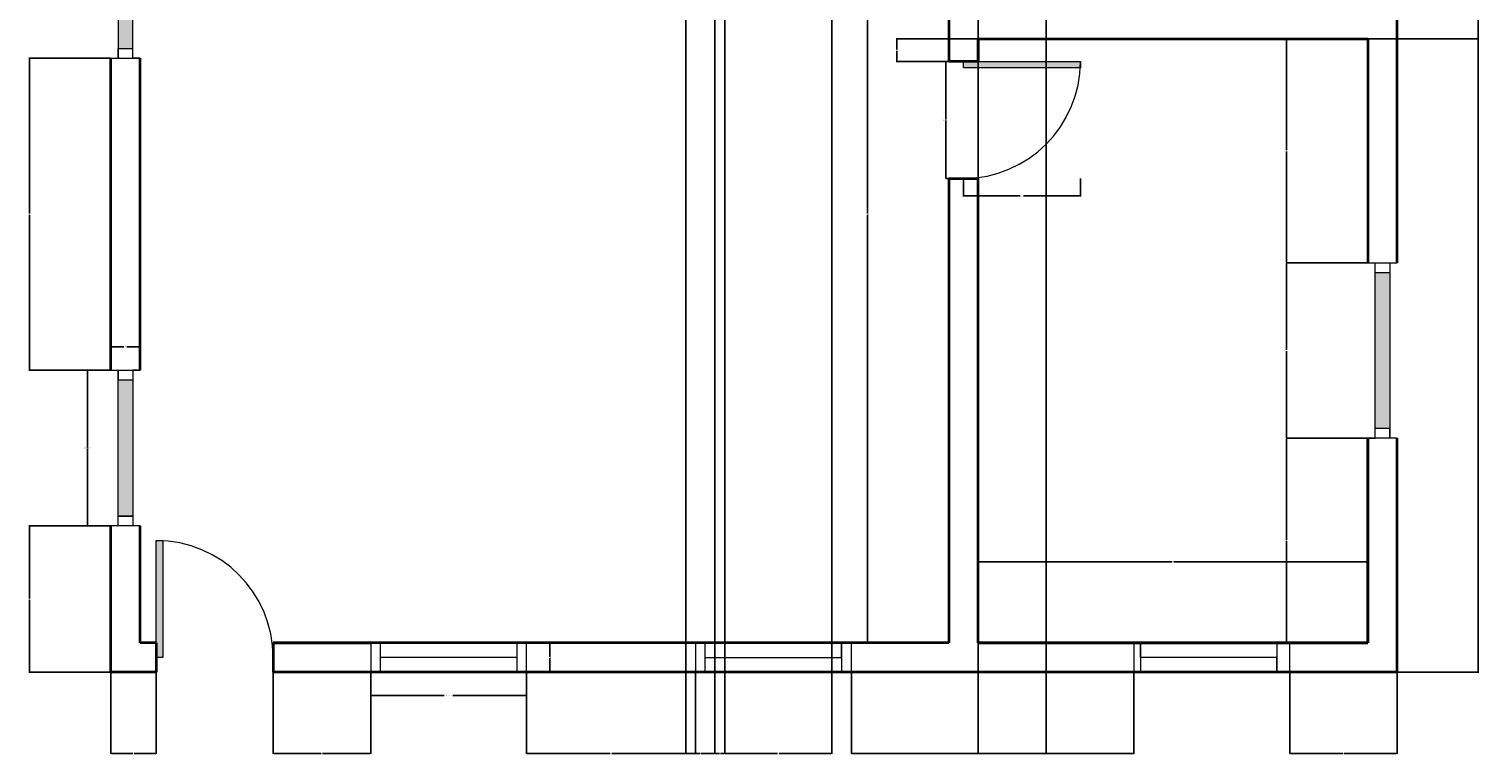
# Model space of a CAD drawing. Units: inches. Extents: x 2039 to 2485, y 1453 to 1986.
# Tile 1 of 4: x 2039 to 2485, y 1453 to 1676. Entities that reach past the tile are written whole.
import ezdxf

# ---------------------------------------------------------------- set-up
doc = ezdxf.new("R2010")
doc.units = ezdxf.units.IN
for name, color, linetype, lineweight in [('A-ANNO-DIMS', 2, 'Continuous', 18), ('A-DOOR', 3, 'Continuous', 18), ('A-GLAZ', 4, 'Continuous', 18), ('A-WALL', 7, 'Continuous', 35)]:
    doc.layers.add(name, color=color, linetype=linetype, lineweight=lineweight)
doc.layers.add('A-OPEN-PATT', color=18, linetype='Continuous', lineweight=13, true_color=0x000000)
doc.styles.get("Standard").update_dxf_attribs({"font": 'arial.ttf'})
doc.dimstyles.get("Standard").update_dxf_attribs({"dimtxt": 0.18, "dimasz": 0.18, "dimexe": 0.18, "dimexo": 0.0625, "dimgap": 0.09, "dimtad": 0, "dimtih": 1, "dimtoh": 1, "dimdec": 4, "dimzin": 0, "dimdsep": 46, "dimtxsty": 'Standard', "dimcen": 0.09, "dimadec": 0, "dimazin": 0, "dimtfac": 1, "dimtdec": 4, "dimtofl": 0, "dimtmove": 0, "dimatfit": 3, "dimfxl": 1, "dimtolj": 1, "dimtzin": 0, "dimarcsym": 0})

# ---------------------------------------------------------------- blocks, each defined once
blk = doc.blocks.new('DOOR-SWING-36IN')
for p, q in [((0, 0), (0, 36)), ((0, 36), (2, 36)), ((2, 36), (2, 0)), ((2, 0), (0, 0))]:
    blk.add_line(p, q)
blk.add_arc((0, 0), 36, 0, 90)
blk = doc.blocks.new('WIN-48IN')
for p, q in [((0, 48), (9, 48)), ((2.25, 3), (2.25, 48)), ((2.25, 48), (2.25, 45)), ((2.25, 45), (6.75, 45)), ((9, 48), (6.75, 48)), ((6.75, 48), (6.75, 0)), ((9, 0), (0, 0)), ((2.25, 0), (2.25, 3)), ((2.25, 3), (6.75, 3)), ((6.75, 3), (2.25, 3)), ((6.75, 0), (2.25, 0))]:
    blk.add_line(p, q)
blk = doc.blocks.new('WIN-48IN-CENTERLINE')
for p, q in [((0, 9), (0, 0)), ((3, 0), (3, 9)), ((45, 9), (45, 0)), ((48, 0), (48, 9)), ((45, 4.5), (3, 4.5))]:
    blk.add_line(p, q)
blk = doc.blocks.new('*D6')
at = {"layer": 'A-ANNO-DIMS', "color": 0, "lineweight": -2, "transparency": 16777216}
for p, q in [((2326.44, 1666.06), (2320.92, 1666.06)), ((2321.1, 1665.88), (2321.1, 1648.24)), ((2321.1, 1630.24), (2321.1, 1647.87)), ((2326.44, 1630.06), (2320.92, 1630.06))]:
    blk.add_line(p, q, dxfattribs=at)
at = {"layer": 'A-ANNO-DIMS', "color": 0, "transparency": 16777216}
for points in [[(2321.07, 1665.88), (2321.13, 1665.88), (2321.1, 1666.06)], [(2321.07, 1630.24), (2321.13, 1630.24), (2321.1, 1630.06)]]:
    blk.add_solid(points, dxfattribs=at)
at = {"layer": 'Defpoints', "color": 0, "transparency": 16777216}
for p in [(2326.5, 1666.06), (2321.1, 1630.06), (2326.5, 1630.06)]:
    blk.add_point(p, dxfattribs=at)
at = {"layer": 'A-ANNO-DIMS', "color": 0, "transparency": 16777216, "insert": (2321.1, 1648.06), "char_height": 0.18, "attachment_point": 5}
blk.add_mtext('\\A1;DOOR D1 36 TYP.', dxfattribs=at)
blk = doc.blocks.new('*D7')
at = {"layer": 'A-ANNO-DIMS', "color": 0, "lineweight": -2, "transparency": 16777216}
for p, q in [((2326.5, 1629.99), (2326.5, 1624.48)), ((2362.5, 1629.99), (2362.5, 1624.48)), ((2326.68, 1624.66), (2343.97, 1624.66)), ((2362.32, 1624.66), (2345.03, 1624.66))]:
    blk.add_line(p, q, dxfattribs=at)
at = {"layer": 'A-ANNO-DIMS', "color": 0, "transparency": 16777216}
for points in [[(2326.68, 1624.69), (2326.68, 1624.63), (2326.5, 1624.66)], [(2362.32, 1624.69), (2362.32, 1624.63), (2362.5, 1624.66)]]:
    blk.add_solid(points, dxfattribs=at)
at = {"layer": 'Defpoints', "color": 0, "transparency": 16777216}
for p in [(2326.5, 1630.06), (2362.5, 1630.06), (2362.5, 1624.66)]:
    blk.add_point(p, dxfattribs=at)
at = {"layer": 'A-ANNO-DIMS', "color": 0, "transparency": 16777216, "insert": (2344.5, 1624.66), "char_height": 0.18, "attachment_point": 5}
blk.add_mtext('\\A1;36 TYP.', dxfattribs=at)
blk = doc.blocks.new('*D12')
at = {"layer": 'A-ANNO-DIMS', "color": 0, "lineweight": -2, "transparency": 16777216}
for p, q in [((2063.94, 1571.06), (2056.62, 1571.06)), ((2056.8, 1570.88), (2056.8, 1547.24)), ((2056.8, 1523.24), (2056.8, 1546.87)), ((2063.94, 1523.06), (2056.62, 1523.06))]:
    blk.add_line(p, q, dxfattribs=at)
at = {"layer": 'A-ANNO-DIMS', "color": 0, "transparency": 16777216}
for points in [[(2056.77, 1570.88), (2056.83, 1570.88), (2056.8, 1571.06)], [(2056.77, 1523.24), (2056.83, 1523.24), (2056.8, 1523.06)]]:
    blk.add_solid(points, dxfattribs=at)
at = {"layer": 'Defpoints', "color": 0, "transparency": 16777216}
for p in [(2056.8, 1571.06), (2064, 1571.06), (2064, 1523.06)]:
    blk.add_point(p, dxfattribs=at)
at = {"layer": 'A-ANNO-DIMS', "color": 0, "transparency": 16777216, "insert": (2056.8, 1547.06), "char_height": 0.18, "attachment_point": 5}
blk.add_mtext('\\A1;WINDOW W2 48 TYP.', dxfattribs=at)
blk = doc.blocks.new('*D13')
at = {"layer": 'A-ANNO-DIMS', "color": 0, "lineweight": -2, "transparency": 16777216}
for p, q in [((2064, 1571.12), (2064, 1578.44)), ((2064.18, 1578.26), (2068.04, 1578.26)), ((2072.82, 1578.26), (2068.96, 1578.26)), ((2073, 1571.12), (2073, 1578.44))]:
    blk.add_line(p, q, dxfattribs=at)
at = {"layer": 'A-ANNO-DIMS', "color": 0, "transparency": 16777216}
for points in [[(2064.18, 1578.29), (2064.18, 1578.23), (2064, 1578.26)], [(2072.82, 1578.29), (2072.82, 1578.23), (2073, 1578.26)]]:
    blk.add_solid(points, dxfattribs=at)
at = {"layer": 'Defpoints', "color": 0, "transparency": 16777216}
for p in [(2073, 1578.26), (2064, 1571.06), (2073, 1571.06)]:
    blk.add_point(p, dxfattribs=at)
at = {"layer": 'A-ANNO-DIMS', "color": 0, "transparency": 16777216, "insert": (2068.5, 1578.26), "char_height": 0.18, "attachment_point": 5}
blk.add_mtext('\\A1;9 TYP.', dxfattribs=at)
blk = doc.blocks.new('*D14')
at = {"layer": 'A-ANNO-DIMS', "color": 0, "lineweight": -2, "transparency": 16777216}
for p, q in [((2144, 1477.99), (2144, 1470.68)), ((2192, 1477.99), (2192, 1470.68)), ((2144.18, 1470.86), (2166.66, 1470.86)), ((2191.82, 1470.86), (2169.34, 1470.86))]:
    blk.add_line(p, q, dxfattribs=at)
at = {"layer": 'A-ANNO-DIMS', "color": 0, "transparency": 16777216}
for points in [[(2144.18, 1470.89), (2144.18, 1470.83), (2144, 1470.86)], [(2191.82, 1470.89), (2191.82, 1470.83), (2192, 1470.86)]]:
    blk.add_solid(points, dxfattribs=at)
at = {"layer": 'Defpoints', "color": 0, "transparency": 16777216}
for p in [(2144, 1478.06), (2192, 1478.06), (2192, 1470.86)]:
    blk.add_point(p, dxfattribs=at)
at = {"layer": 'A-ANNO-DIMS', "color": 0, "transparency": 16777216, "insert": (2168, 1470.86), "char_height": 0.18, "attachment_point": 5}
blk.add_mtext('\\A1;WINDOW W3 48 TYP.', dxfattribs=at)
blk = doc.blocks.new('*D15')
at = {"layer": 'A-ANNO-DIMS', "color": 0, "lineweight": -2, "transparency": 16777216}
for p, q in [((2192.06, 1487.06), (2199.38, 1487.06)), ((2199.2, 1486.88), (2199.2, 1482.74)), ((2199.2, 1478.24), (2199.2, 1482.37)), ((2192.06, 1478.06), (2199.38, 1478.06))]:
    blk.add_line(p, q, dxfattribs=at)
at = {"layer": 'A-ANNO-DIMS', "color": 0, "transparency": 16777216}
for points in [[(2199.17, 1486.88), (2199.23, 1486.88), (2199.2, 1487.06)], [(2199.17, 1478.24), (2199.23, 1478.24), (2199.2, 1478.06)]]:
    blk.add_solid(points, dxfattribs=at)
at = {"layer": 'Defpoints', "color": 0, "transparency": 16777216}
for p in [(2192, 1487.06), (2199.2, 1487.06), (2192, 1478.06)]:
    blk.add_point(p, dxfattribs=at)
at = {"layer": 'A-ANNO-DIMS', "color": 0, "transparency": 16777216, "insert": (2199.2, 1482.56), "char_height": 0.18, "attachment_point": 5}
blk.add_mtext('\\A1;9 TYP.', dxfattribs=at)
blk = doc.blocks.new('*D17')
at = {"layer": 'A-ANNO-DIMS', "color": 0, "lineweight": -2, "transparency": 16777216}
for p, q in [((2460.06, 1961.06), (2485.19, 1961.06)), ((2485.01, 1960.88), (2485.01, 1719.74)), ((2485.01, 1478.24), (2485.01, 1719.37)), ((2460.06, 1478.06), (2485.19, 1478.06))]:
    blk.add_line(p, q, dxfattribs=at)
at = {"layer": 'A-ANNO-DIMS', "color": 0, "transparency": 16777216}
for points in [[(2484.98, 1960.88), (2485.04, 1960.88), (2485.01, 1961.06)], [(2484.98, 1478.24), (2485.04, 1478.24), (2485.01, 1478.06)]]:
    blk.add_solid(points, dxfattribs=at)
at = {"layer": 'Defpoints', "color": 0, "transparency": 16777216}
for p in [(2460, 1961.06), (2460, 1478.06), (2485.01, 1478.06)]:
    blk.add_point(p, dxfattribs=at)
at = {"layer": 'A-ANNO-DIMS', "color": 0, "transparency": 16777216, "insert": (2485.01, 1719.56), "char_height": 0.18, "attachment_point": 5}
blk.add_mtext('\\A1;483', dxfattribs=at)
blk = doc.blocks.new('*D20')
at = {"layer": 'A-ANNO-DIMS', "color": 0, "lineweight": -2, "transparency": 16777216}
for p, q in [((2064, 1477.99), (2064, 1452.87)), ((2078, 1477.99), (2078, 1452.87)), ((2064.18, 1453.05), (2070.79, 1453.05)), ((2077.82, 1453.05), (2071.21, 1453.05))]:
    blk.add_line(p, q, dxfattribs=at)
at = {"layer": 'A-ANNO-DIMS', "color": 0, "transparency": 16777216}
for points in [[(2064.18, 1453.08), (2064.18, 1453.02), (2064, 1453.05)], [(2077.82, 1453.08), (2077.82, 1453.02), (2078, 1453.05)]]:
    blk.add_solid(points, dxfattribs=at)
at = {"layer": 'Defpoints', "color": 0, "transparency": 16777216}
for p in [(2064, 1478.06), (2078, 1478.06), (2078, 1453.05)]:
    blk.add_point(p, dxfattribs=at)
at = {"layer": 'A-ANNO-DIMS', "color": 0, "transparency": 16777216, "insert": (2071, 1453.05), "char_height": 0.18, "attachment_point": 5}
blk.add_mtext('\\A1;14', dxfattribs=at)
blk = doc.blocks.new('*D21')
at = {"layer": 'A-ANNO-DIMS', "color": 0, "lineweight": -2, "transparency": 16777216}
for p, q in [((2114, 1477.99), (2114, 1452.87)), ((2144, 1477.99), (2144, 1452.87)), ((2114.18, 1453.05), (2128.78, 1453.05)), ((2143.82, 1453.05), (2129.22, 1453.05))]:
    blk.add_line(p, q, dxfattribs=at)
at = {"layer": 'A-ANNO-DIMS', "color": 0, "transparency": 16777216}
for points in [[(2114.18, 1453.08), (2114.18, 1453.02), (2114, 1453.05)], [(2143.82, 1453.08), (2143.82, 1453.02), (2144, 1453.05)]]:
    blk.add_solid(points, dxfattribs=at)
at = {"layer": 'Defpoints', "color": 0, "transparency": 16777216}
for p in [(2114, 1478.06), (2144, 1478.06), (2144, 1453.05)]:
    blk.add_point(p, dxfattribs=at)
at = {"layer": 'A-ANNO-DIMS', "color": 0, "transparency": 16777216, "insert": (2129, 1453.05), "char_height": 0.18, "attachment_point": 5}
blk.add_mtext('\\A1;30', dxfattribs=at)
blk = doc.blocks.new('*D22')
at = {"layer": 'A-ANNO-DIMS', "color": 0, "lineweight": -2, "transparency": 16777216}
for p, q in [((2192, 1477.99), (2192, 1452.87)), ((2244, 1477.99), (2244, 1452.87)), ((2192.18, 1453.05), (2217.78, 1453.05)), ((2243.82, 1453.05), (2218.22, 1453.05))]:
    blk.add_line(p, q, dxfattribs=at)
at = {"layer": 'A-ANNO-DIMS', "color": 0, "transparency": 16777216}
for points in [[(2192.18, 1453.08), (2192.18, 1453.02), (2192, 1453.05)], [(2243.82, 1453.08), (2243.82, 1453.02), (2244, 1453.05)]]:
    blk.add_solid(points, dxfattribs=at)
at = {"layer": 'Defpoints', "color": 0, "transparency": 16777216}
for p in [(2192, 1478.06), (2244, 1478.06), (2244, 1453.05)]:
    blk.add_point(p, dxfattribs=at)
at = {"layer": 'A-ANNO-DIMS', "color": 0, "transparency": 16777216, "insert": (2218, 1453.05), "char_height": 0.18, "attachment_point": 5}
blk.add_mtext('\\A1;52', dxfattribs=at)
blk = doc.blocks.new('*D23')
at = {"layer": 'A-ANNO-DIMS', "color": 0, "lineweight": -2, "transparency": 16777216}
for p, q in [((2292, 1477.99), (2292, 1452.87)), ((2379, 1477.99), (2379, 1452.87)), ((2292.18, 1453.05), (2335.28, 1453.05)), ((2378.82, 1453.05), (2335.72, 1453.05))]:
    blk.add_line(p, q, dxfattribs=at)
at = {"layer": 'A-ANNO-DIMS', "color": 0, "transparency": 16777216}
for points in [[(2292.18, 1453.08), (2292.18, 1453.02), (2292, 1453.05)], [(2378.82, 1453.08), (2378.82, 1453.02), (2379, 1453.05)]]:
    blk.add_solid(points, dxfattribs=at)
at = {"layer": 'Defpoints', "color": 0, "transparency": 16777216}
for p in [(2292, 1478.06), (2379, 1478.06), (2379, 1453.05)]:
    blk.add_point(p, dxfattribs=at)
at = {"layer": 'A-ANNO-DIMS', "color": 0, "transparency": 16777216, "insert": (2335.5, 1453.05), "char_height": 0.18, "attachment_point": 5}
blk.add_mtext('\\A1;87', dxfattribs=at)
blk = doc.blocks.new('*D24')
at = {"layer": 'A-ANNO-DIMS', "color": 0, "lineweight": -2, "transparency": 16777216}
for p, q in [((2427, 1477.99), (2427, 1452.87)), ((2460, 1477.99), (2460, 1452.87)), ((2427.18, 1453.05), (2443.28, 1453.05)), ((2459.82, 1453.05), (2443.72, 1453.05))]:
    blk.add_line(p, q, dxfattribs=at)
at = {"layer": 'A-ANNO-DIMS', "color": 0, "transparency": 16777216}
for points in [[(2427.18, 1453.08), (2427.18, 1453.02), (2427, 1453.05)], [(2459.82, 1453.08), (2459.82, 1453.02), (2460, 1453.05)]]:
    blk.add_solid(points, dxfattribs=at)
at = {"layer": 'Defpoints', "color": 0, "transparency": 16777216}
for p in [(2427, 1478.06), (2460, 1478.06), (2460, 1453.05)]:
    blk.add_point(p, dxfattribs=at)
at = {"layer": 'A-ANNO-DIMS', "color": 0, "transparency": 16777216, "insert": (2443.5, 1453.05), "char_height": 0.18, "attachment_point": 5}
blk.add_mtext('\\A1;33', dxfattribs=at)
blk = doc.blocks.new('*D25')
at = {"layer": 'A-ANNO-DIMS', "color": 0, "lineweight": -2, "transparency": 16777216}
for p, q in [((2063.94, 1523.06), (2038.81, 1523.06)), ((2038.99, 1522.88), (2038.99, 1500.74)), ((2038.99, 1478.24), (2038.99, 1500.37)), ((2063.94, 1478.06), (2038.81, 1478.06))]:
    blk.add_line(p, q, dxfattribs=at)
at = {"layer": 'A-ANNO-DIMS', "color": 0, "transparency": 16777216}
for points in [[(2038.96, 1522.88), (2039.02, 1522.88), (2038.99, 1523.06)], [(2038.96, 1478.24), (2039.02, 1478.24), (2038.99, 1478.06)]]:
    blk.add_solid(points, dxfattribs=at)
at = {"layer": 'Defpoints', "color": 0, "transparency": 16777216}
for p in [(2038.99, 1523.06), (2064, 1523.06), (2064, 1478.06)]:
    blk.add_point(p, dxfattribs=at)
at = {"layer": 'A-ANNO-DIMS', "color": 0, "transparency": 16777216, "insert": (2038.99, 1500.56), "char_height": 0.18, "attachment_point": 5}
blk.add_mtext('\\A1;45', dxfattribs=at)
blk = doc.blocks.new('*D26')
at = {"layer": 'A-ANNO-DIMS', "color": 0, "lineweight": -2, "transparency": 16777216}
for p, q in [((2063.94, 1667.06), (2038.81, 1667.06)), ((2038.99, 1666.88), (2038.99, 1619.24)), ((2038.99, 1571.24), (2038.99, 1618.87)), ((2063.94, 1571.06), (2038.81, 1571.06))]:
    blk.add_line(p, q, dxfattribs=at)
at = {"layer": 'A-ANNO-DIMS', "color": 0, "transparency": 16777216}
for points in [[(2038.96, 1666.88), (2039.02, 1666.88), (2038.99, 1667.06)], [(2038.96, 1571.24), (2039.02, 1571.24), (2038.99, 1571.06)]]:
    blk.add_solid(points, dxfattribs=at)
at = {"layer": 'Defpoints', "color": 0, "transparency": 16777216}
for p in [(2038.99, 1667.06), (2064, 1667.06), (2064, 1571.06)]:
    blk.add_point(p, dxfattribs=at)
at = {"layer": 'A-ANNO-DIMS', "color": 0, "transparency": 16777216, "insert": (2038.99, 1619.06), "char_height": 0.18, "attachment_point": 5}
blk.add_mtext('\\A1;96', dxfattribs=at)
blk = doc.blocks.new('*D29')
at = {"layer": 'A-ANNO-DIMS', "color": 0, "lineweight": -2, "transparency": 16777216}
for p, q in [((2450.94, 1550.06), (2425.81, 1550.06)), ((2425.99, 1549.88), (2425.99, 1518.74)), ((2425.99, 1487.24), (2425.99, 1518.37)), ((2450.94, 1487.06), (2425.81, 1487.06))]:
    blk.add_line(p, q, dxfattribs=at)
at = {"layer": 'A-ANNO-DIMS', "color": 0, "transparency": 16777216}
for points in [[(2425.96, 1549.88), (2426.02, 1549.88), (2425.99, 1550.06)], [(2425.96, 1487.24), (2426.02, 1487.24), (2425.99, 1487.06)]]:
    blk.add_solid(points, dxfattribs=at)
at = {"layer": 'Defpoints', "color": 0, "transparency": 16777216}
for p in [(2425.99, 1550.06), (2451, 1550.06), (2451, 1487.06)]:
    blk.add_point(p, dxfattribs=at)
at = {"layer": 'A-ANNO-DIMS', "color": 0, "transparency": 16777216, "insert": (2425.99, 1518.56), "char_height": 0.18, "attachment_point": 5}
blk.add_mtext('\\A1;63', dxfattribs=at)
blk = doc.blocks.new('*D30')
at = {"layer": 'A-ANNO-DIMS', "color": 0, "lineweight": -2, "transparency": 16777216}
for p, q in [((2450.94, 1604.06), (2425.81, 1604.06)), ((2425.99, 1603.88), (2425.99, 1577.24)), ((2425.99, 1550.24), (2425.99, 1576.87)), ((2450.94, 1550.06), (2425.81, 1550.06))]:
    blk.add_line(p, q, dxfattribs=at)
at = {"layer": 'A-ANNO-DIMS', "color": 0, "transparency": 16777216}
for points in [[(2425.96, 1603.88), (2426.02, 1603.88), (2425.99, 1604.06)], [(2425.96, 1550.24), (2426.02, 1550.24), (2425.99, 1550.06)]]:
    blk.add_solid(points, dxfattribs=at)
at = {"layer": 'Defpoints', "color": 0, "transparency": 16777216}
for p in [(2425.99, 1604.06), (2451, 1604.06), (2451, 1550.06)]:
    blk.add_point(p, dxfattribs=at)
at = {"layer": 'A-ANNO-DIMS', "color": 0, "transparency": 16777216, "insert": (2425.99, 1577.06), "char_height": 0.18, "attachment_point": 5}
blk.add_mtext('\\A1;54', dxfattribs=at)
blk = doc.blocks.new('*D31')
at = {"layer": 'A-ANNO-DIMS', "color": 0, "lineweight": -2, "transparency": 16777216}
for p, q in [((2450.94, 1673.06), (2425.81, 1673.06)), ((2425.99, 1672.88), (2425.99, 1638.74)), ((2425.99, 1604.24), (2425.99, 1638.37)), ((2450.94, 1604.06), (2425.81, 1604.06))]:
    blk.add_line(p, q, dxfattribs=at)
at = {"layer": 'A-ANNO-DIMS', "color": 0, "transparency": 16777216}
for points in [[(2425.96, 1672.88), (2426.02, 1672.88), (2425.99, 1673.06)], [(2425.96, 1604.24), (2426.02, 1604.24), (2425.99, 1604.06)]]:
    blk.add_solid(points, dxfattribs=at)
at = {"layer": 'Defpoints', "color": 0, "transparency": 16777216}
for p in [(2425.99, 1673.06), (2451, 1673.06), (2451, 1604.06)]:
    blk.add_point(p, dxfattribs=at)
at = {"layer": 'A-ANNO-DIMS', "color": 0, "transparency": 16777216, "insert": (2425.99, 1638.56), "char_height": 0.18, "attachment_point": 5}
blk.add_mtext('\\A1;69', dxfattribs=at)
blk = doc.blocks.new('*D36')
at = {"layer": 'A-ANNO-DIMS', "color": 0, "lineweight": -2, "transparency": 16777216}
for p, q in [((2330.939914, 1673.056109), (2305.811914, 1673.056109)), ((2305.991914, 1672.876109), (2305.991914, 1669.736109)), ((2330.939914, 1666.056109), (2305.811914, 1666.056109)), ((2305.991914, 1666.236109), (2305.991914, 1669.376109))]:
    blk.add_line(p, q, dxfattribs=at)
at = {"layer": 'A-ANNO-DIMS', "color": 0, "transparency": 16777216}
for points in [[(2305.961914, 1672.876109), (2306.021914, 1672.876109), (2305.991914, 1673.056109)], [(2305.961914, 1666.236109), (2306.021914, 1666.236109), (2305.991914, 1666.056109)]]:
    blk.add_solid(points, dxfattribs=at)
at = {"layer": 'Defpoints', "color": 0, "transparency": 16777216}
for p in [(2305.991914, 1673.056109), (2331.002414, 1673.056109), (2331.002414, 1666.056109)]:
    blk.add_point(p, dxfattribs=at)
at = {"layer": 'A-ANNO-DIMS', "color": 0, "transparency": 16777216, "insert": (2305.991914, 1669.556109), "char_height": 0.18, "attachment_point": 5}
blk.add_mtext('\\A1;7', dxfattribs=at)
blk = doc.blocks.new('*D40')
at = {"layer": 'A-ANNO-DIMS', "color": 0, "lineweight": -2, "transparency": 16777216}
for p, q in [((2321.94, 1751.06), (2296.81, 1751.06)), ((2296.99, 1750.88), (2296.99, 1619.24)), ((2296.99, 1487.24), (2296.99, 1618.87)), ((2321.94, 1487.06), (2296.81, 1487.06))]:
    blk.add_line(p, q, dxfattribs=at)
at = {"layer": 'A-ANNO-DIMS', "color": 0, "transparency": 16777216}
for points in [[(2296.96, 1750.88), (2297.02, 1750.88), (2296.99, 1751.06)], [(2296.96, 1487.24), (2297.02, 1487.24), (2296.99, 1487.06)]]:
    blk.add_solid(points, dxfattribs=at)
at = {"layer": 'Defpoints', "color": 0, "transparency": 16777216}
for p in [(2296.99, 1751.06), (2322, 1751.06), (2322, 1487.06)]:
    blk.add_point(p, dxfattribs=at)
at = {"layer": 'A-ANNO-DIMS', "color": 0, "transparency": 16777216, "insert": (2296.99, 1619.06), "char_height": 0.18, "attachment_point": 5}
blk.add_mtext('\\A1;264', dxfattribs=at)
blk = doc.blocks.new('*D41')
at = {"layer": 'A-ANNO-DIMS', "color": 0, "lineweight": -2, "transparency": 16777216}
for p, q in [((2331, 1487.12), (2331, 1512.25)), ((2331.18, 1512.07), (2390.72, 1512.07)), ((2450.82, 1512.07), (2391.28, 1512.07)), ((2451, 1487.12), (2451, 1512.25))]:
    blk.add_line(p, q, dxfattribs=at)
at = {"layer": 'A-ANNO-DIMS', "color": 0, "transparency": 16777216}
for points in [[(2331.18, 1512.1), (2331.18, 1512.04), (2331, 1512.07)], [(2450.82, 1512.1), (2450.82, 1512.04), (2451, 1512.07)]]:
    blk.add_solid(points, dxfattribs=at)
at = {"layer": 'Defpoints', "color": 0, "transparency": 16777216}
for p in [(2451, 1512.07), (2331, 1487.06), (2451, 1487.06)]:
    blk.add_point(p, dxfattribs=at)
at = {"layer": 'A-ANNO-DIMS', "color": 0, "transparency": 16777216, "insert": (2391, 1512.07), "char_height": 0.18, "attachment_point": 5}
blk.add_mtext('\\A1;120', dxfattribs=at)
blk = doc.blocks.new('*D42')
at = {"layer": 'A-ANNO-DIMS', "color": 0, "lineweight": -2, "transparency": 16777216}
for p, q in [((2241, 1759.99), (2241, 1452.87)), ((2250, 1759.99), (2250, 1452.87)), ((2241.18, 1453.05), (2245.35, 1453.05)), ((2249.82, 1453.05), (2245.65, 1453.05))]:
    blk.add_line(p, q, dxfattribs=at)
at = {"layer": 'A-ANNO-DIMS', "color": 0, "transparency": 16777216}
for points in [[(2241.18, 1453.08), (2241.18, 1453.02), (2241, 1453.05)], [(2249.82, 1453.08), (2249.82, 1453.02), (2250, 1453.05)]]:
    blk.add_solid(points, dxfattribs=at)
at = {"layer": 'Defpoints', "color": 0, "transparency": 16777216}
for p in [(2241, 1760.06), (2250, 1760.06), (2250, 1453.05)]:
    blk.add_point(p, dxfattribs=at)
at = {"layer": 'A-ANNO-DIMS', "color": 0, "transparency": 16777216, "insert": (2245.5, 1453.05), "char_height": 0.18, "attachment_point": 5}
blk.add_mtext('\\A1;9', dxfattribs=at)
blk = doc.blocks.new('*D54')
at = {"layer": 'A-ANNO-DIMS', "color": 0, "lineweight": -2, "transparency": 16777216}
for p, q in [((2250, 1759.99), (2250, 1452.87)), ((2253, 1750.99), (2253, 1452.87)), ((2250.18, 1453.05), (2251.35, 1453.05)), ((2252.82, 1453.05), (2251.65, 1453.05))]:
    blk.add_line(p, q, dxfattribs=at)
at = {"layer": 'A-ANNO-DIMS', "color": 0, "transparency": 16777216}
for points in [[(2250.18, 1453.08), (2250.18, 1453.02), (2250, 1453.05)], [(2252.82, 1453.08), (2252.82, 1453.02), (2253, 1453.05)]]:
    blk.add_solid(points, dxfattribs=at)
at = {"layer": 'Defpoints', "color": 0, "transparency": 16777216}
for p in [(2250, 1760.06), (2253, 1751.06), (2253, 1453.05)]:
    blk.add_point(p, dxfattribs=at)
at = {"layer": 'A-ANNO-DIMS', "color": 0, "transparency": 16777216, "insert": (2251.5, 1453.05), "char_height": 0.18, "attachment_point": 5}
blk.add_mtext('\\A1;3', dxfattribs=at)
blk = doc.blocks.new('*D55')
at = {"layer": 'A-ANNO-DIMS', "color": 0, "lineweight": -2, "transparency": 16777216}
for p, q in [((2253, 1750.99), (2253, 1452.87)), ((2286, 1750.99), (2286, 1452.87)), ((2253.18, 1453.05), (2269.28, 1453.05)), ((2285.82, 1453.05), (2269.72, 1453.05))]:
    blk.add_line(p, q, dxfattribs=at)
at = {"layer": 'A-ANNO-DIMS', "color": 0, "transparency": 16777216}
for points in [[(2253.18, 1453.08), (2253.18, 1453.02), (2253, 1453.05)], [(2285.82, 1453.08), (2285.82, 1453.02), (2286, 1453.05)]]:
    blk.add_solid(points, dxfattribs=at)
at = {"layer": 'Defpoints', "color": 0, "transparency": 16777216}
for p in [(2253, 1751.06), (2286, 1751.06), (2286, 1453.05)]:
    blk.add_point(p, dxfattribs=at)
at = {"layer": 'A-ANNO-DIMS', "color": 0, "transparency": 16777216, "insert": (2269.5, 1453.05), "char_height": 0.18, "attachment_point": 5}
blk.add_mtext('\\A1;33', dxfattribs=at)
blk = doc.blocks.new('*D58')
at = {"layer": 'A-ANNO-DIMS', "color": 0, "lineweight": -2, "transparency": 16777216}
for p, q in [((2331, 1678.99), (2331, 1452.87)), ((2352, 1678.99), (2352, 1452.87)), ((2331.18, 1453.05), (2341.3, 1453.05)), ((2351.82, 1453.05), (2341.71, 1453.05))]:
    blk.add_line(p, q, dxfattribs=at)
at = {"layer": 'A-ANNO-DIMS', "color": 0, "transparency": 16777216}
for points in [[(2331.18, 1453.08), (2331.18, 1453.02), (2331, 1453.05)], [(2351.82, 1453.08), (2351.82, 1453.02), (2352, 1453.05)]]:
    blk.add_solid(points, dxfattribs=at)
at = {"layer": 'Defpoints', "color": 0, "transparency": 16777216}
for p in [(2331, 1679.06), (2352, 1679.06), (2352, 1453.05)]:
    blk.add_point(p, dxfattribs=at)
at = {"layer": 'A-ANNO-DIMS', "color": 0, "transparency": 16777216, "insert": (2341.5, 1453.05), "char_height": 0.18, "attachment_point": 5}
blk.add_mtext('\\A1;21', dxfattribs=at)
blk = doc.blocks.new('*D65')
at = {"layer": 'A-ANNO-DIMS', "color": 0, "lineweight": -2, "transparency": 16777216}
for p, q in [((2451.06, 1679.06), (2485.19, 1679.06)), ((2485.01, 1678.88), (2485.01, 1676.24)), ((2485.01, 1673.24), (2485.01, 1675.87)), ((2451.06, 1673.06), (2485.19, 1673.06))]:
    blk.add_line(p, q, dxfattribs=at)
at = {"layer": 'A-ANNO-DIMS', "color": 0, "transparency": 16777216}
for points in [[(2484.98, 1678.88), (2485.04, 1678.88), (2485.01, 1679.06)], [(2484.98, 1673.24), (2485.04, 1673.24), (2485.01, 1673.06)]]:
    blk.add_solid(points, dxfattribs=at)
at = {"layer": 'Defpoints', "color": 0, "transparency": 16777216}
for p in [(2451, 1679.06), (2485.01, 1679.06), (2451, 1673.06)]:
    blk.add_point(p, dxfattribs=at)
at = {"layer": 'A-ANNO-DIMS', "color": 0, "transparency": 16777216, "insert": (2485.01, 1676.06), "char_height": 0.18, "attachment_point": 5}
blk.add_mtext('\\A1;6', dxfattribs=at)

msp = doc.modelspace()

# ---------------------------------------------------------------- hatches: boundary and pattern name
at = {"layer": 'A-OPEN-PATT'}
h = msp.add_hatch(color=256, dxfattribs=at)
h.dxf.hatch_style = 1
h.paths.add_polyline_path([(2070.75, 1853.06), (2066.25, 1853.06), (2066.25, 1799.06), (2070.75, 1799.06)])
h.paths.add_polyline_path([(2080, 1791.5, 0.013897), (2078, 1791.56), (2078, 1755.56), (2080, 1755.56)])
h.paths.add_polyline_path([(2070.75, 1712.06), (2066.25, 1712.06), (2066.25, 1670.06), (2070.75, 1670.06)])
h.paths.add_polyline_path([(2070.75, 1568.06), (2066.25, 1568.06), (2066.25, 1526.06), (2070.75, 1526.06)])
h.paths.add_polyline_path([(2080, 1518.5, 0.013897), (2078, 1518.56), (2078, 1482.56), (2080, 1482.56)])
h.paths.add_polyline_path([(2362.5, 1666.06), (2326.5, 1666.06), (2326.5, 1664.06), (2362.45, 1664.06, 0.013897)])
h.paths.add_polyline_path([(2457.75, 1601.06), (2453.25, 1601.06), (2453.25, 1553.06), (2457.75, 1553.06)])
h.paths.add_polyline_path([(2457.75, 1799.06), (2453.25, 1799.06), (2453.25, 1769.06), (2457.75, 1769.06)])
h.paths.add_polyline_path([(2336, 1791.5, 0.013897), (2334, 1791.56), (2334, 1755.56), (2336, 1755.56)])
h.paths.add_polyline_path([(2255, 1788.5, 0.015162), (2253, 1788.56), (2253, 1755.56), (2255, 1755.56)])
h.paths.add_polyline_path([(2331, 1830.06), (2322, 1830.06), (2322, 1828.06), (2331, 1828.06)])
h.paths.add_polyline_path([(2250, 1896.06), (2245.5, 1896.06), (2241, 1896.06), (2241, 1894.06), (2250, 1894.06)])
h.paths.add_polyline_path([(2271.5, 1896.06), (2250, 1896.06), (2250, 1894.06), (2271.5, 1894.06)])
h.paths.add_polyline_path([(2304, 1958.81), (2268, 1958.81), (2268, 1954.31), (2304, 1954.31)])

# ---------------------------------------------------------------- linework, layer by layer
at = {"layer": 'A-GLAZ'}
for p, q in [((2451, 1604.06), (2460, 1604.06)), ((2453.25, 1550.06), (2453.25, 1604.06)), ((2453.25, 1604.06), (2457.75, 1604.06)), ((2457.75, 1604.06), (2457.75, 1550.06)), ((2453.25, 1553.06), (2453.25, 1601.06)), ((2453.25, 1601.06), (2457.75, 1601.06)), ((2460, 1550.06), (2451, 1550.06)), ((2451, 1550.06), (2453.25, 1550.06)), ((2457.75, 1553.06), (2453.25, 1553.06)), ((2457.75, 1550.06), (2457.75, 1553.06)), ((2147, 1487.06), (2171, 1487.06)), ((2180, 1487.06), (2177, 1487.06)), ((2244, 1487.06), (2247, 1487.06)), ((2289, 1482.56), (2289, 1487.06)), ((2379, 1487.06), (2379, 1478.06)), ((2381, 1482.56), (2381, 1487.06)), ((2381, 1487.06), (2381, 1478.06)), ((2424, 1487.06), (2423, 1487.06)), ((2423, 1487.06), (2423, 1478.06)), ((2427, 1487.06), (2424, 1487.06)), ((2427, 1478.06), (2427, 1487.06)), ((2247, 1478.06), (2247, 1482.56)), ((2423, 1482.56), (2381, 1482.56)), ((2423, 1478.06), (2423, 1482.56)), ((2144, 1478.06), (2147, 1478.06)), ((2144, 1478.06), (2180, 1478.06)), ((2171, 1478.06), (2174, 1478.06)), ((2256, 1478.06), (2244, 1478.06)), ((2292, 1478.06), (2256, 1478.06)), ((2379, 1478.06), (2427, 1478.06))]:
    msp.add_line(p, q, dxfattribs=at)
at = {"layer": 'A-WALL'}
for p, q in [((2322, 1751.06), (2322, 1666.06)), ((2460, 1604.06), (2460, 1751.06)), ((2331, 1673.06), (2451, 1673.06)), ((2331, 1673.06), (2331, 1666.06)), ((2331, 1666.06), (2331, 1673.06)), ((2451, 1673.06), (2451, 1604.06)), ((2451, 1673.06), (2451, 1604.06)), ((2064, 1571.06), (2064, 1667.06)), ((2073, 1571.06), (2073, 1667.06)), ((2331, 1666.06), (2322, 1666.06)), ((2322, 1630.06), (2331, 1630.06)), ((2322, 1630.06), (2322, 1487.06)), ((2331, 1487.06), (2331, 1630.06)), ((2451, 1487.06), (2451, 1550.06)), ((2451, 1550.06), (2451, 1487.06)), ((2451, 1550.06), (2451, 1487.06)), ((2460, 1478.06), (2460, 1550.06)), ((2064, 1478.06), (2064, 1523.06)), ((2073, 1487.06), (2073, 1523.06)), ((2073, 1487.06), (2073, 1523.06)), ((2078, 1487.06), (2073, 1487.06)), ((2078, 1487.06), (2078, 1478.06)), ((2322, 1487.06), (2114, 1487.06)), ((2114, 1487.06), (2114, 1478.06)), ((2114, 1487.06), (2144, 1487.06)), ((2322, 1487.06), (2292, 1487.06)), ((2451, 1487.06), (2331, 1487.06)), ((2331, 1487.06), (2451, 1487.06)), ((2391, 1487.06), (2379, 1487.06)), ((2451, 1487.06), (2391, 1487.06)), ((2078, 1478.06), (2064, 1478.06)), ((2460, 1478.06), (2114, 1478.06))]:
    msp.add_line(p, q, dxfattribs=at)

# ---------------------------------------------------------------- block references
at = {"layer": 'A-DOOR', "rotation": 269.9999999999995}
msp.add_blockref('DOOR-SWING-36IN', (2326.5, 1666.06), dxfattribs=at)
at = {"layer": 'A-DOOR'}
msp.add_blockref('DOOR-SWING-36IN', (2078, 1482.56), dxfattribs=at)
at = {"layer": 'A-GLAZ', "extrusion": (0, 0, -1), "zscale": -1, "rotation": 180}
msp.add_blockref('WIN-48IN', (-2064, 1715.06), dxfattribs=at)
at = {"layer": 'A-GLAZ'}
for name, p in [('WIN-48IN', (2064, 1523.06)), ('WIN-48IN-CENTERLINE', (2144, 1478.06))]:
    msp.add_blockref(name, p, dxfattribs=at)
at = {"layer": 'A-GLAZ', "rotation": 180}
msp.add_blockref('WIN-48IN-CENTERLINE', (2292, 1487.06), dxfattribs=at)

# ---------------------------------------------------------------- dimensions: what is measured, and where the dimension line sits
at = {"layer": 'A-ANNO-DIMS'}
for base, p1, p2, angle, picture, middle in [((2485.01, 1478.06), (2460, 1961.06), (2460, 1478.06), 270, '*D17', (2485.01, 1719.56)), ((2296.99, 1751.06), (2322, 1487.06), (2322, 1751.06), 90, '*D40', (2296.99, 1619.06)), ((2485.01, 1679.06), (2451, 1673.06), (2451, 1679.06), 90, '*D65', (2485.01, 1676.06)), ((2305.99, 1673.06), (2331, 1666.06), (2331, 1673.06), 90, '*D36', (2305.99, 1669.56)), ((2425.99, 1673.06), (2451, 1604.06), (2451, 1673.06), 90, '*D31', (2425.99, 1638.56)), ((2038.99, 1667.06), (2064, 1571.06), (2064, 1667.06), 90, '*D26', (2038.99, 1619.06)), ((2425.99, 1604.06), (2451, 1550.06), (2451, 1604.06), 90, '*D30', (2425.99, 1577.06)), ((2425.99, 1550.06), (2451, 1487.06), (2451, 1550.06), 90, '*D29', (2425.99, 1518.56)), ((2038.99, 1523.06), (2064, 1478.06), (2064, 1523.06), 90, '*D25', (2038.99, 1500.56))]:
    dim = msp.add_linear_dim(base=base, p1=p1, p2=p2, angle=angle, dimstyle='Standard', override={"dimdec": 0, "dimlfac": 1, "dimrnd": 0, "dimzin": 0, "dimdsep": 46, "dimlunit": 2}, dxfattribs=at)
    dim.commit()
    dim.dimension.update_dxf_attribs({"geometry": picture, "text_midpoint": middle})
for base, p1, p2, picture, middle in [((2250, 1453.05), (2241, 1760.06), (2250, 1760.06), '*D42', (2245.5, 1453.05)), ((2253, 1453.05), (2250, 1760.06), (2253, 1751.06), '*D54', (2251.5, 1453.05)), ((2286, 1453.05), (2253, 1751.06), (2286, 1751.06), '*D55', (2269.5, 1453.05)), ((2352, 1453.05), (2331, 1679.06), (2352, 1679.06), '*D58', (2341.5, 1453.05)), ((2451, 1512.07), (2331, 1487.06), (2451, 1487.06), '*D41', (2391, 1512.07)), ((2078, 1453.05), (2064, 1478.06), (2078, 1478.06), '*D20', (2071, 1453.05)), ((2144, 1453.05), (2114, 1478.06), (2144, 1478.06), '*D21', (2129, 1453.05)), ((2244, 1453.05), (2192, 1478.06), (2244, 1478.06), '*D22', (2218, 1453.05)), ((2379, 1453.05), (2292, 1478.06), (2379, 1478.06), '*D23', (2335.5, 1453.05)), ((2460, 1453.05), (2427, 1478.06), (2460, 1478.06), '*D24', (2443.5, 1453.05))]:
    dim = msp.add_linear_dim(base=base, p1=p1, p2=p2, dimstyle='Standard', override={"dimdec": 0, "dimlfac": 1, "dimrnd": 0, "dimzin": 0, "dimdsep": 46, "dimlunit": 2}, dxfattribs=at)
    dim.commit()
    dim.dimension.update_dxf_attribs({"geometry": picture, "text_midpoint": middle})
for base, p1, p2, angle, text, picture, middle in [((2321.1, 1630.06), (2326.5, 1666.06), (2326.5, 1630.06), 270, 'DOOR D1 <> TYP.', '*D6', (2321.1, 1648.06)), ((2056.8, 1571.06), (2064, 1523.06), (2064, 1571.06), 90, 'WINDOW W2 <> TYP.', '*D12', (2056.8, 1547.06)), ((2199.2, 1487.06), (2192, 1478.06), (2192, 1487.06), 90, '<> TYP.', '*D15', (2199.2, 1482.56))]:
    dim = msp.add_linear_dim(base=base, p1=p1, p2=p2, angle=angle, text=text, dimstyle='Standard', override={"dimdec": 0, "dimlfac": 1, "dimrnd": 0, "dimzin": 0, "dimdsep": 46, "dimlunit": 2}, dxfattribs=at)
    dim.commit()
    dim.dimension.update_dxf_attribs({"geometry": picture, "text_midpoint": middle})
for base, p1, p2, text, picture, middle in [((2362.5, 1624.66), (2326.5, 1630.06), (2362.5, 1630.06), '<> TYP.', '*D7', (2344.5, 1624.66)), ((2073, 1578.26), (2064, 1571.06), (2073, 1571.06), '<> TYP.', '*D13', (2068.5, 1578.26)), ((2192, 1470.86), (2144, 1478.06), (2192, 1478.06), 'WINDOW W3 <> TYP.', '*D14', (2168, 1470.86))]:
    dim = msp.add_linear_dim(base=base, p1=p1, p2=p2, text=text, dimstyle='Standard', override={"dimdec": 0, "dimlfac": 1, "dimrnd": 0, "dimzin": 0, "dimdsep": 46, "dimlunit": 2}, dxfattribs=at)
    dim.commit()
    dim.dimension.update_dxf_attribs({"geometry": picture, "text_midpoint": middle})

doc.saveas('drawing.dxf')
